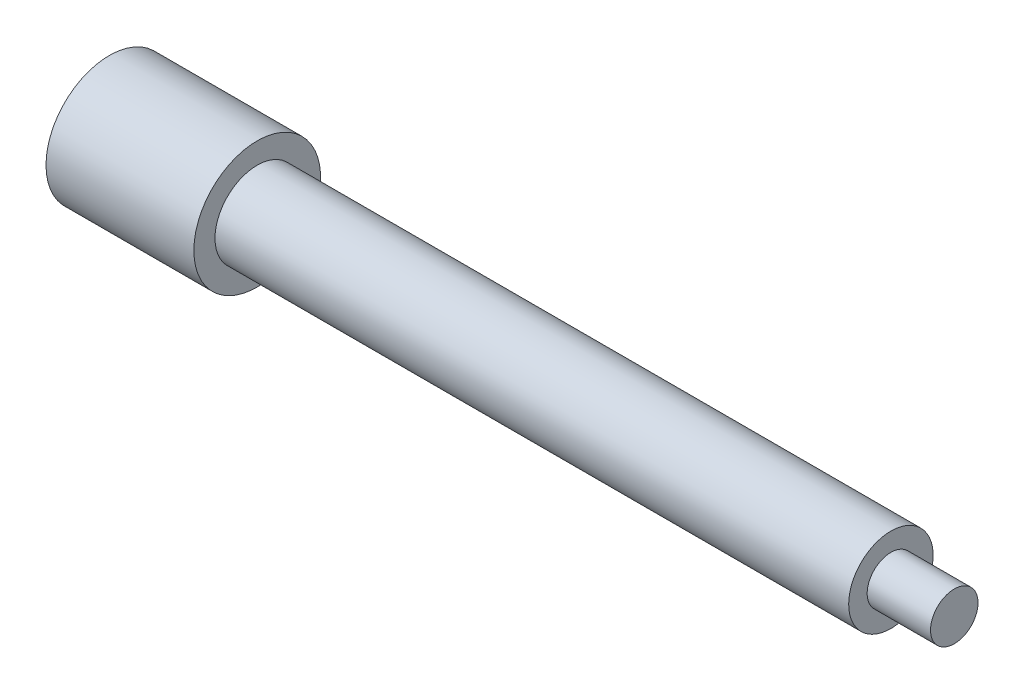
SolidWorks part; units mm, degrees
material "Plain Carbon Steel"
ref_plane "Front Plane" through (0, 0, 0) normal (0, 0, 1) x (1, 0, 0)
ref_plane "Top Plane" through (0, 0, 0) normal (0, 1, 0) x (1, 0, 0)
ref_plane "Right Plane" through (0, 0, 0) normal (1, 0, 0) x (0, 0, -1)
sketch "Stepped Shaft Profile" plane through (0, 0, 0) normal (0, 0, 1) x (1, 0, 0)
  line L0 (0, 0) -> (0, 6)
  line L1 (0, 6) -> (14, 6)
  line L2 (14, 6) -> (14, 4)
  line L3 (14, 4) -> (74, 4)
  line L5 (0, 0) -> (80, 0)
  line L6 (74, 4) -> (74, 2.25)
  line L7 (74, 2.25) -> (80, 2.25)
  line L8 (80, 2.25) -> (80, 0)
  dimension "D1" = 14
  dimension "D2" = 6
  dimension "D3" = 4
  dimension "D4" = 2.25
  dimension "D5" = 6
  dimension "D6" = 80
revolve "Stepped Shaft Revolve" add sketch "Stepped Shaft Profile" angle 360 about L5
